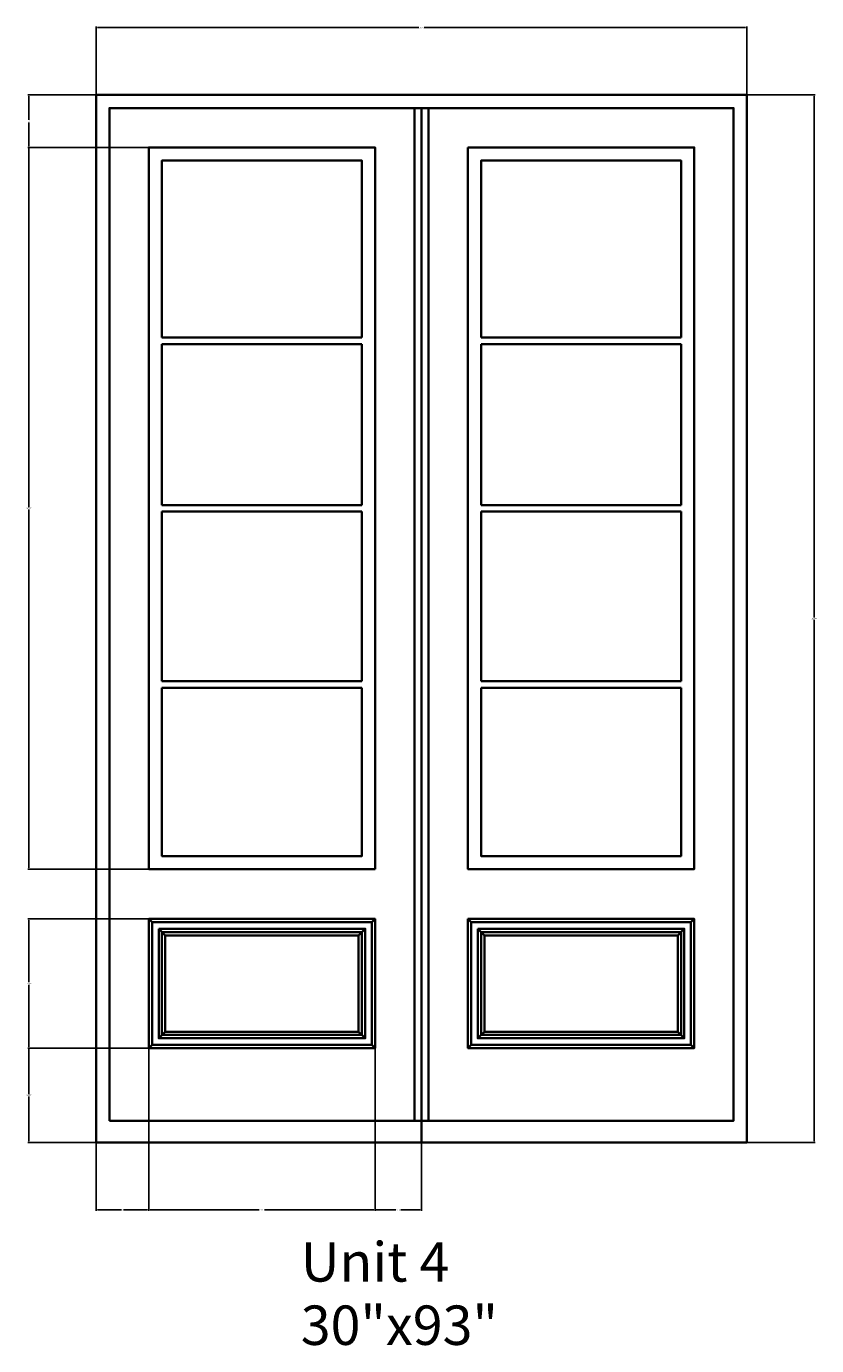
# Model space of a CAD drawing. Units: inches. Extents: x 1318 to 1980, y 617 to 1423.
# Tile 7 of 7: x 1681 to 1801, y 1222 to 1423. Entities that reach past the tile are written whole.
import ezdxf

# ---------------------------------------------------------------- set-up
doc = ezdxf.new("R2010")
doc.units = ezdxf.units.IN
doc.header["$MEASUREMENT"] = 0
for name, color, linetype, lineweight in [('A-ANNO-DIMS', 2, 'Continuous', 18), ('A-ANNO-TEXT', 7, 'Continuous', 25), ('A-DOOR', 4, 'Continuous', 35)]:
    doc.layers.add(name, color=color, linetype=linetype, lineweight=lineweight)
doc.styles.get("Standard").update_dxf_attribs({"font": 'arial.ttf'})
doc.dimstyles.get("Standard").update_dxf_attribs({"dimtxt": 0.18, "dimasz": 0.18, "dimexe": 0.18, "dimexo": 0.0625, "dimgap": 0.09, "dimtad": 0, "dimtih": 1, "dimtoh": 1, "dimdec": 0, "dimzin": 0, "dimdsep": 46, "dimlunit": 3, "dimtxsty": 'Standard', "dimcen": 0.09, "dimadec": 0, "dimazin": 0, "dimtfac": 1, "dimtdec": 0, "dimtofl": 0, "dimtmove": 0, "dimatfit": 3, "dimfxl": 1, "dimtolj": 1, "dimtzin": 0, "dimarcsym": 0})

# ---------------------------------------------------------------- blocks, each defined once
blk = doc.blocks.new('*D23')
at = {"layer": 'A-ANNO-DIMS', "color": 0, "lineweight": -2, "transparency": 16777216}
for p, q in [((1691.16, 1412.68), (1691.16, 1423.04)), ((1691.34, 1422.86), (1740.25, 1422.86)), ((1789.95, 1422.86), (1741.04, 1422.86)), ((1790.13, 1412.68), (1790.13, 1423.04))]:
    blk.add_line(p, q, dxfattribs=at)
at = {"layer": 'A-ANNO-DIMS', "color": 0, "transparency": 16777216}
for points in [[(1691.34, 1422.89), (1691.34, 1422.83), (1691.16, 1422.86)], [(1789.95, 1422.89), (1789.95, 1422.83), (1790.13, 1422.86)]]:
    blk.add_solid(points, dxfattribs=at)
at = {"layer": 'Defpoints', "color": 0, "transparency": 16777216}
for p in [(1790.13, 1422.86), (1691.16, 1412.61), (1790.13, 1412.61)]:
    blk.add_point(p, dxfattribs=at)
at = {"layer": 'A-ANNO-DIMS', "color": 0, "transparency": 16777216, "insert": (1740.64, 1422.86), "char_height": 0.18, "attachment_point": 5}
blk.add_mtext('\\A1;98.98', dxfattribs=at)
blk = doc.blocks.new('*D24')
at = {"layer": 'A-ANNO-DIMS', "color": 0, "lineweight": -2, "transparency": 16777216}
for p, q in [((1790.2, 1412.61), (1800.56, 1412.61)), ((1800.38, 1412.43), (1800.38, 1333.06)), ((1800.38, 1253.32), (1800.38, 1332.7)), ((1790.2, 1253.14), (1800.56, 1253.14))]:
    blk.add_line(p, q, dxfattribs=at)
at = {"layer": 'A-ANNO-DIMS', "color": 0, "transparency": 16777216}
for points in [[(1800.35, 1412.43), (1800.41, 1412.43), (1800.38, 1412.61)], [(1800.35, 1253.32), (1800.41, 1253.32), (1800.38, 1253.14)]]:
    blk.add_solid(points, dxfattribs=at)
at = {"layer": 'Defpoints', "color": 0, "transparency": 16777216}
for p in [(1790.13, 1412.61), (1800.38, 1412.61), (1790.13, 1253.14)]:
    blk.add_point(p, dxfattribs=at)
at = {"layer": 'A-ANNO-DIMS', "color": 0, "transparency": 16777216, "insert": (1800.38, 1332.88), "char_height": 0.18, "attachment_point": 5}
blk.add_mtext('\\A1;159.47', dxfattribs=at)
blk = doc.blocks.new('*D25')
at = {"layer": 'A-ANNO-DIMS', "color": 0, "lineweight": -2, "transparency": 16777216}
for p, q in [((1699.16, 1267.44), (1699.16, 1242.71)), ((1691.16, 1253.08), (1691.16, 1242.71)), ((1691.34, 1242.89), (1695.01, 1242.89)), ((1698.98, 1242.89), (1695.3, 1242.89))]:
    blk.add_line(p, q, dxfattribs=at)
at = {"layer": 'A-ANNO-DIMS', "color": 0, "transparency": 16777216}
for points in [[(1691.34, 1242.92), (1691.34, 1242.86), (1691.16, 1242.89)], [(1698.98, 1242.92), (1698.98, 1242.86), (1699.16, 1242.89)]]:
    blk.add_solid(points, dxfattribs=at)
at = {"layer": 'Defpoints', "color": 0, "transparency": 16777216}
for p in [(1699.16, 1267.5), (1691.16, 1253.14), (1699.16, 1242.89)]:
    blk.add_point(p, dxfattribs=at)
at = {"layer": 'A-ANNO-DIMS', "color": 0, "transparency": 16777216, "insert": (1695.16, 1242.89), "char_height": 0.18, "attachment_point": 5}
blk.add_mtext('\\A1;8', dxfattribs=at)
blk = doc.blocks.new('*D26')
at = {"layer": 'A-ANNO-DIMS', "color": 0, "lineweight": -2, "transparency": 16777216}
for p, q in [((1699.16, 1267.44), (1699.16, 1242.71)), ((1733.58, 1267.44), (1733.58, 1242.71)), ((1699.34, 1242.89), (1715.97, 1242.89)), ((1733.4, 1242.89), (1716.76, 1242.89))]:
    blk.add_line(p, q, dxfattribs=at)
at = {"layer": 'A-ANNO-DIMS', "color": 0, "transparency": 16777216}
for points in [[(1699.34, 1242.92), (1699.34, 1242.86), (1699.16, 1242.89)], [(1733.4, 1242.92), (1733.4, 1242.86), (1733.58, 1242.89)]]:
    blk.add_solid(points, dxfattribs=at)
at = {"layer": 'Defpoints', "color": 0, "transparency": 16777216}
for p in [(1699.16, 1267.5), (1733.58, 1267.5), (1733.58, 1242.89)]:
    blk.add_point(p, dxfattribs=at)
at = {"layer": 'A-ANNO-DIMS', "color": 0, "transparency": 16777216, "insert": (1716.37, 1242.89), "char_height": 0.18, "attachment_point": 5}
blk.add_mtext('\\A1;34.42', dxfattribs=at)
blk = doc.blocks.new('*D27')
at = {"layer": 'A-ANNO-DIMS', "color": 0, "lineweight": -2, "transparency": 16777216}
for p, q in [((1733.58, 1267.44), (1733.58, 1242.71)), ((1740.64, 1253.08), (1740.64, 1242.71)), ((1733.76, 1242.89), (1736.72, 1242.89)), ((1740.46, 1242.89), (1737.5, 1242.89))]:
    blk.add_line(p, q, dxfattribs=at)
at = {"layer": 'A-ANNO-DIMS', "color": 0, "transparency": 16777216}
for points in [[(1733.76, 1242.92), (1733.76, 1242.86), (1733.58, 1242.89)], [(1740.46, 1242.92), (1740.46, 1242.86), (1740.64, 1242.89)]]:
    blk.add_solid(points, dxfattribs=at)
at = {"layer": 'Defpoints', "color": 0, "transparency": 16777216}
for p in [(1733.58, 1267.5), (1740.64, 1253.14), (1740.64, 1242.89)]:
    blk.add_point(p, dxfattribs=at)
at = {"layer": 'A-ANNO-DIMS', "color": 0, "transparency": 16777216, "insert": (1737.11, 1242.89), "char_height": 0.18, "attachment_point": 5}
blk.add_mtext('\\A1;7.068', dxfattribs=at)
blk = doc.blocks.new('*D28')
at = {"layer": 'A-ANNO-DIMS', "color": 0, "lineweight": -2, "transparency": 16777216}
for p, q in [((1699.09, 1267.5), (1680.73, 1267.5)), ((1680.91, 1267.32), (1680.91, 1260.5)), ((1680.91, 1253.32), (1680.91, 1260.14)), ((1691.09, 1253.14), (1680.73, 1253.14))]:
    blk.add_line(p, q, dxfattribs=at)
at = {"layer": 'A-ANNO-DIMS', "color": 0, "transparency": 16777216}
for points in [[(1680.88, 1267.32), (1680.94, 1267.32), (1680.91, 1267.5)], [(1680.88, 1253.32), (1680.94, 1253.32), (1680.91, 1253.14)]]:
    blk.add_solid(points, dxfattribs=at)
at = {"layer": 'Defpoints', "color": 0, "transparency": 16777216}
for p in [(1680.91, 1267.5), (1699.16, 1267.5), (1691.16, 1253.14)]:
    blk.add_point(p, dxfattribs=at)
at = {"layer": 'A-ANNO-DIMS', "color": 0, "transparency": 16777216, "insert": (1680.91, 1260.32), "char_height": 0.18, "attachment_point": 5}
blk.add_mtext('\\A1;14.357', dxfattribs=at)
blk = doc.blocks.new('*D29')
at = {"layer": 'A-ANNO-DIMS', "color": 0, "lineweight": -2, "transparency": 16777216}
for p, q in [((1699.09, 1287.17), (1680.73, 1287.17)), ((1680.91, 1286.99), (1680.91, 1277.52)), ((1680.91, 1267.68), (1680.91, 1277.15)), ((1699.09, 1267.5), (1680.73, 1267.5))]:
    blk.add_line(p, q, dxfattribs=at)
at = {"layer": 'A-ANNO-DIMS', "color": 0, "transparency": 16777216}
for points in [[(1680.88, 1286.99), (1680.94, 1286.99), (1680.91, 1287.17)], [(1680.88, 1267.68), (1680.94, 1267.68), (1680.91, 1267.5)]]:
    blk.add_solid(points, dxfattribs=at)
at = {"layer": 'Defpoints', "color": 0, "transparency": 16777216}
for p in [(1680.91, 1287.17), (1699.16, 1287.17), (1699.16, 1267.5)]:
    blk.add_point(p, dxfattribs=at)
at = {"layer": 'A-ANNO-DIMS', "color": 0, "transparency": 16777216, "insert": (1680.91, 1277.33), "char_height": 0.18, "attachment_point": 5}
blk.add_mtext('\\A1;19.664', dxfattribs=at)
blk = doc.blocks.new('*D30')
at = {"layer": 'A-ANNO-DIMS', "color": 0, "lineweight": -2, "transparency": 16777216}
for p, q in [((1699.09, 1404.61), (1680.73, 1404.61)), ((1680.91, 1404.43), (1680.91, 1349.86)), ((1680.91, 1294.93), (1680.91, 1349.5)), ((1699.09, 1294.75), (1680.73, 1294.75))]:
    blk.add_line(p, q, dxfattribs=at)
at = {"layer": 'A-ANNO-DIMS', "color": 0, "transparency": 16777216}
for points in [[(1680.88, 1404.43), (1680.94, 1404.43), (1680.91, 1404.61)], [(1680.88, 1294.93), (1680.94, 1294.93), (1680.91, 1294.75)]]:
    blk.add_solid(points, dxfattribs=at)
at = {"layer": 'Defpoints', "color": 0, "transparency": 16777216}
for p in [(1680.91, 1404.61), (1699.16, 1404.61), (1699.16, 1294.75)]:
    blk.add_point(p, dxfattribs=at)
at = {"layer": 'A-ANNO-DIMS', "color": 0, "transparency": 16777216, "insert": (1680.91, 1349.68), "char_height": 0.18, "attachment_point": 5}
blk.add_mtext('\\A1;109.87', dxfattribs=at)
blk = doc.blocks.new('*D31')
at = {"layer": 'A-ANNO-DIMS', "color": 0, "lineweight": -2, "transparency": 16777216}
for p, q in [((1691.09, 1412.61), (1680.73, 1412.61)), ((1680.91, 1412.43), (1680.91, 1408.8)), ((1680.91, 1404.79), (1680.91, 1408.43)), ((1699.09, 1404.61), (1680.73, 1404.61))]:
    blk.add_line(p, q, dxfattribs=at)
at = {"layer": 'A-ANNO-DIMS', "color": 0, "transparency": 16777216}
for points in [[(1680.88, 1412.43), (1680.94, 1412.43), (1680.91, 1412.61)], [(1680.88, 1404.79), (1680.94, 1404.79), (1680.91, 1404.61)]]:
    blk.add_solid(points, dxfattribs=at)
at = {"layer": 'Defpoints', "color": 0, "transparency": 16777216}
for p in [(1680.91, 1412.61), (1691.16, 1412.61), (1699.16, 1404.61)]:
    blk.add_point(p, dxfattribs=at)
at = {"layer": 'A-ANNO-DIMS', "color": 0, "transparency": 16777216, "insert": (1680.91, 1408.61), "char_height": 0.18, "attachment_point": 5}
blk.add_mtext('\\A1;8', dxfattribs=at)

msp = doc.modelspace()

# ---------------------------------------------------------------- linework, layer by layer
at = {"layer": 'A-DOOR'}
for p, q in [((1739.5765, 1256.4377), (1739.5765, 1410.615)), ((1740.6445, 1256.4377), (1740.6445, 1410.615)), ((1741.7125, 1256.4377), (1741.7125, 1410.615)), ((1701.1552, 1375.6684), (1731.5765, 1375.6684)), ((1701.1552, 1374.6684), (1731.5765, 1374.6684)), ((1716.7955, 1375.6684), (1731.5765, 1375.6684)), ((1716.7955, 1374.6684), (1731.5765, 1374.6684)), ((1749.7125, 1375.6684), (1780.1337, 1375.6684)), ((1749.7125, 1374.6684), (1780.1337, 1374.6684)), ((1765.3527, 1375.6684), (1780.1337, 1375.6684)), ((1765.3527, 1374.6684), (1780.1337, 1374.6684)), ((1701.1552, 1350.1824), (1731.5765, 1350.1824)), ((1716.7955, 1350.1824), (1731.5765, 1350.1824)), ((1749.7125, 1350.1824), (1780.1337, 1350.1824)), ((1765.3527, 1350.1824), (1780.1337, 1350.1824)), ((1701.1552, 1349.1824), (1731.5765, 1349.1824)), ((1716.7955, 1349.1824), (1731.5765, 1349.1824)), ((1749.7125, 1349.1824), (1780.1337, 1349.1824)), ((1765.3527, 1349.1824), (1780.1337, 1349.1824)), ((1701.1552, 1323.3594), (1731.5765, 1323.3594)), ((1701.1552, 1322.3594), (1731.5765, 1322.3594)), ((1716.7955, 1323.3594), (1731.5765, 1323.3594)), ((1716.7955, 1322.3594), (1731.5765, 1322.3594)), ((1749.7125, 1323.3594), (1780.1337, 1323.3594)), ((1749.7125, 1322.3594), (1780.1337, 1322.3594)), ((1765.3527, 1323.3594), (1780.1337, 1323.3594)), ((1765.3527, 1322.3594), (1780.1337, 1322.3594)), ((1699.1552, 1287.1657), (1699.6552, 1286.6657)), ((1700.6552, 1285.6657), (1701.6552, 1284.6657)), ((1731.0765, 1284.6657), (1732.0765, 1285.6657)), ((1733.0765, 1286.6657), (1733.5765, 1287.1657)), ((1747.7125, 1287.1657), (1748.2125, 1286.6657)), ((1749.2125, 1285.6657), (1750.2125, 1284.6657)), ((1779.6337, 1284.6657), (1780.6337, 1285.6657)), ((1781.6337, 1286.6657), (1782.1337, 1287.1657)), ((1700.6552, 1269.0015), (1701.6552, 1270.0015)), ((1732.0765, 1269.0015), (1731.0765, 1270.0015)), ((1749.2125, 1269.0015), (1750.2125, 1270.0015)), ((1780.6337, 1269.0015), (1779.6337, 1270.0015)), ((1699.1552, 1267.5015), (1699.6552, 1268.0015)), ((1733.5765, 1267.5015), (1733.0765, 1268.0015)), ((1747.7125, 1267.5015), (1748.2125, 1268.0015)), ((1782.1337, 1267.5015), (1781.6337, 1268.0015)), ((1740.6445, 1256.4377), (1740.6445, 1253.1444))]:
    msp.add_line(p, q, dxfattribs=at)
for points in [[(1691.1552, 1412.615), (1790.1337, 1412.615), (1790.1337, 1253.1444), (1691.1552, 1253.1444)], [(1693.1552, 1256.4377), (1693.1552, 1410.615), (1788.1337, 1410.615), (1788.1337, 1256.4377)], [(1733.5765, 1294.7497), (1699.1552, 1294.7497), (1699.1552, 1404.615), (1733.5765, 1404.615)], [(1747.7125, 1404.615), (1782.1337, 1404.615), (1782.1337, 1294.7497), (1747.7125, 1294.7497)], [(1699.1552, 1287.1657), (1733.5765, 1287.1657), (1733.5765, 1267.5015), (1699.1552, 1267.5015)], [(1699.6552, 1286.6657), (1733.0765, 1286.6657), (1733.0765, 1268.0015), (1699.6552, 1268.0015)], [(1700.6552, 1285.6657), (1732.0765, 1285.6657), (1732.0765, 1269.0015), (1700.6552, 1269.0015)], [(1747.7125, 1287.1657), (1782.1337, 1287.1657), (1782.1337, 1267.5015), (1747.7125, 1267.5015)], [(1748.2125, 1286.6657), (1781.6337, 1286.6657), (1781.6337, 1268.0015), (1748.2125, 1268.0015)], [(1749.2125, 1285.6657), (1780.6337, 1285.6657), (1780.6337, 1269.0015), (1749.2125, 1269.0015)], [(1701.1552, 1285.1657), (1731.5765, 1285.1657), (1731.5765, 1269.5015), (1701.1552, 1269.5015)], [(1701.6552, 1284.6657), (1731.0765, 1284.6657), (1731.0765, 1270.0015), (1701.6552, 1270.0015)], [(1749.7125, 1285.1657), (1780.1337, 1285.1657), (1780.1337, 1269.5015), (1749.7125, 1269.5015)], [(1750.2125, 1284.6657), (1779.6337, 1284.6657), (1779.6337, 1270.0015), (1750.2125, 1270.0015)]]:
    msp.add_lwpolyline(points, close=True, dxfattribs=at)
for points in [[(1701.1552, 1375.6684), (1701.1552, 1402.615), (1731.5765, 1402.615), (1731.5765, 1375.6684)], [(1749.7125, 1375.6684), (1749.7125, 1402.615), (1780.1337, 1402.615), (1780.1337, 1375.6684)], [(1701.1552, 1350.1824), (1701.1552, 1374.6684)], [(1731.5765, 1374.6684), (1731.5765, 1350.1824)], [(1749.7125, 1350.1824), (1749.7125, 1374.6684)], [(1780.1337, 1374.6684), (1780.1337, 1350.1824)], [(1701.1552, 1323.3594), (1701.1552, 1349.1824)], [(1731.5765, 1349.1824), (1731.5765, 1323.3594)], [(1749.7125, 1323.3594), (1749.7125, 1349.1824)], [(1780.1337, 1349.1824), (1780.1337, 1323.3594)], [(1731.5765, 1322.3594), (1731.5765, 1296.7497), (1701.1552, 1296.7497), (1701.1552, 1322.3594)], [(1780.1337, 1322.3594), (1780.1337, 1296.7497), (1749.7125, 1296.7497), (1749.7125, 1322.3594)]]:
    msp.add_lwpolyline(points, dxfattribs=at)

# ---------------------------------------------------------------- texts
at = {"layer": 'A-ANNO-TEXT'}
for s, p in [('Unit 4', (1722.2726, 1231.9597)), ('30"x93"', (1722.2726, 1222.3213))]:
    msp.add_text(s, height=6, dxfattribs=at).set_placement(p)

# ---------------------------------------------------------------- dimensions: what is measured, and where the dimension line sits
at = {"layer": 'A-ANNO-DIMS'}
for base, p1, p2, override, picture, middle in [((1790.1337, 1422.865), (1691.1552, 1412.615), (1790.1337, 1412.615), {"dimdec": 2, "dimlfac": 1, "dimrnd": 0, "dimzin": 0, "dimdsep": 46, "dimlunit": 2}, '*D23', (1740.6445, 1422.865)), ((1699.1552, 1242.8944), (1691.1552, 1253.1444), (1699.1552, 1267.5015), {"dimdec": 0, "dimlfac": 1, "dimrnd": 0, "dimzin": 0, "dimdsep": 46, "dimlunit": 2}, '*D25', (1695.1552, 1242.8944)), ((1733.5765, 1242.8944), (1699.1552, 1267.5015), (1733.5765, 1267.5015), {"dimdec": 2, "dimlfac": 1, "dimrnd": 0, "dimzin": 0, "dimdsep": 46, "dimlunit": 2}, '*D26', (1716.3659, 1242.8944)), ((1740.6445, 1242.8944), (1733.5765, 1267.5015), (1740.6445, 1253.1444), {"dimdec": 3, "dimlfac": 1, "dimrnd": 0, "dimzin": 0, "dimdsep": 46, "dimlunit": 2}, '*D27', (1737.1105, 1242.8944))]:
    dim = msp.add_linear_dim(base=base, p1=p1, p2=p2, dimstyle='Standard', override=override, dxfattribs=at)
    dim.commit()
    dim.dimension.update_dxf_attribs({"geometry": picture, "text_midpoint": middle})
for base, p1, p2, override, picture, middle in [((1680.9052, 1412.615), (1699.1552, 1404.615), (1691.1552, 1412.615), {"dimdec": 0, "dimlfac": 1, "dimrnd": 0, "dimzin": 0, "dimdsep": 46, "dimlunit": 2}, '*D31', (1680.9052, 1408.615)), ((1800.3837, 1412.615), (1790.1337, 1253.1444), (1790.1337, 1412.615), {"dimdec": 2, "dimlfac": 1, "dimrnd": 0, "dimzin": 0, "dimdsep": 46, "dimlunit": 2}, '*D24', (1800.3837, 1332.8797)), ((1680.9052, 1404.615), (1699.1552, 1294.7497), (1699.1552, 1404.615), {"dimdec": 2, "dimlfac": 1, "dimrnd": 0, "dimzin": 0, "dimdsep": 46, "dimlunit": 2}, '*D30', (1680.9052, 1349.6824)), ((1680.9052, 1287.1657), (1699.1552, 1267.5015), (1699.1552, 1287.1657), {"dimdec": 3, "dimlfac": 1, "dimrnd": 0, "dimzin": 0, "dimdsep": 46, "dimlunit": 2}, '*D29', (1680.9052, 1277.3336)), ((1680.9052, 1267.5015), (1691.1552, 1253.1444), (1699.1552, 1267.5015), {"dimdec": 3, "dimlfac": 1, "dimrnd": 0, "dimzin": 0, "dimdsep": 46, "dimlunit": 2}, '*D28', (1680.9052, 1260.323))]:
    dim = msp.add_linear_dim(base=base, p1=p1, p2=p2, angle=90, dimstyle='Standard', override=override, dxfattribs=at)
    dim.commit()
    dim.dimension.update_dxf_attribs({"geometry": picture, "text_midpoint": middle})

doc.saveas('drawing.dxf')
